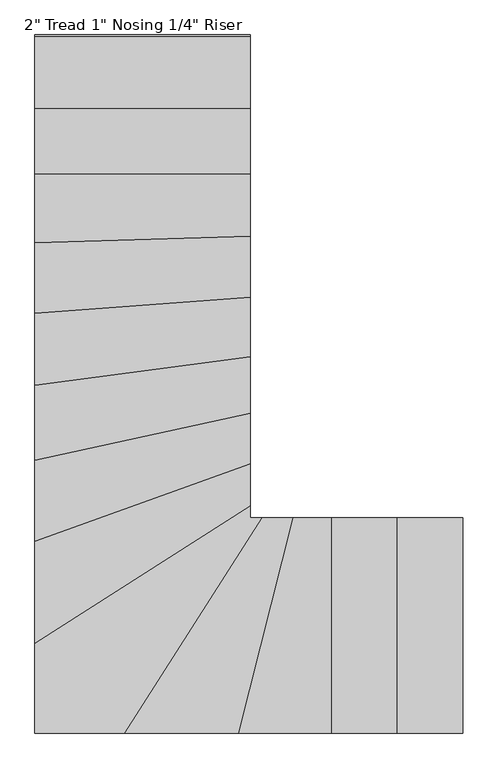
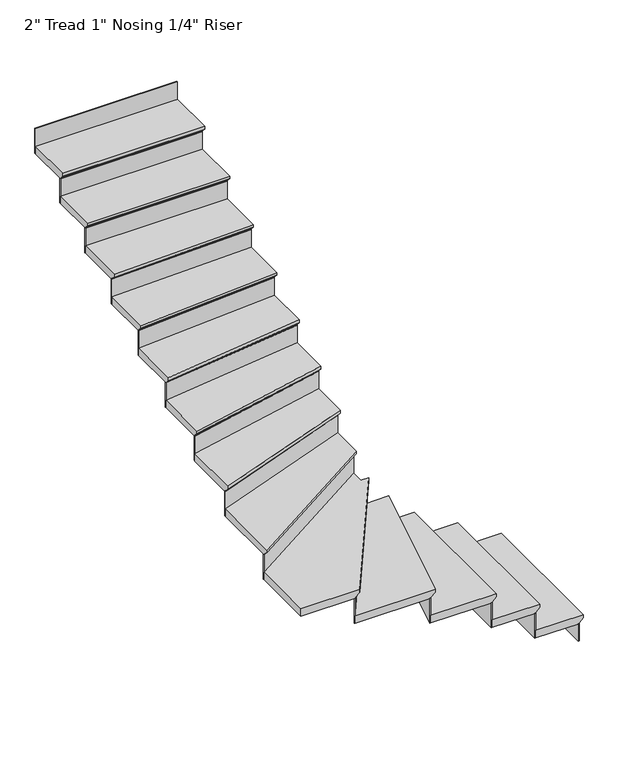
"""IFC4 building model written with IfcOpenShell, lengths in millimetres: stair flight geometry."""

from ifc_helpers import new_model, si_unit, origin, place, context, project, spatial, faceted_brep, source, transform, mapped, element, save


def stair_flight_c47d8ec9(model_context):
    return source(origin(), model_context, "Body", "Brep", [
        faceted_brep([(-4378.4230036, -1246.1564015, 827.6166667), (-4378.4230036, -1246.1564015, 846.6666667), (-4378.4230036, -2160.5564015, 846.6666667), (-4378.4230036, -2160.5564015, 827.6166667), (-4403.8230036, -1246.1564015, 802.2166667), (-4403.8230036, -2160.5564015, 802.2166667), (-4683.2230036, -1246.1564015, 846.6666667), (-4683.2230036, -2160.5564015, 846.6666667), (-4403.8230036, -2160.5564015, 795.8666667), (-4683.2230036, -2160.5564015, 795.8666667), (-4683.2230036, -1246.1564015, 795.8666667), (-4403.8230036, -1246.1564015, 795.8666667)], [[[0, 1, 2, 3]], [[4, 0, 3, 5]], [[2, 1, 6, 7]], [[8, 9, 10, 11]], [[2, 7, 9, 8, 5, 3]], [[8, 11, 4, 5]], [[6, 1, 0, 4, 11, 10]], [[7, 6, 10, 9]]]),
        faceted_brep([(-4403.8230036, -1246.1564015, 795.8666667), (-4403.8230036, -1246.1564015, 677.3333333), (-4410.1730036, -1246.1564015, 677.3333333), (-4410.1730036, -1246.1564015, 795.8666667), (-4403.8230036, -2160.5564015, 795.8666667), (-4410.1730036, -2160.5564015, 795.8666667), (-4410.1730036, -2160.5564015, 677.3333333), (-4403.8230036, -2160.5564015, 677.3333333)], [[[0, 1, 2, 3]], [[4, 5, 6, 7]], [[1, 0, 4, 7]], [[2, 1, 7, 6]], [[3, 2, 6, 5]], [[0, 3, 5, 4]]]),
        faceted_brep([(-4683.2230036, -1246.1564015, 965.2), (-4683.2230036, -1246.1564015, 795.8666667), (-4689.5730036, -1246.1564015, 795.8666667), (-4689.5730036, -1246.1564015, 965.2), (-4683.2230036, -2160.5564015, 965.2), (-4689.5730036, -2160.5564015, 965.2), (-4689.5730036, -2160.5564015, 795.8666667), (-4683.2230036, -2160.5564015, 795.8666667)], [[[0, 1, 2, 3]], [[4, 5, 6, 7]], [[1, 0, 4, 7]], [[2, 1, 7, 6]], [[3, 2, 6, 5]], [[0, 3, 5, 4]]]),
        faceted_brep([(-4657.8230036, -2160.5564015, 1016.0), (-4657.8230036, -1246.1564015, 1016.0), (-4962.6230036, -1246.1564015, 1016.0), (-4962.6230036, -2160.5564015, 1016.0), (-4683.2230036, -2160.5564015, 965.2), (-4962.6230036, -2160.5564015, 965.2), (-4962.6230036, -1246.1564015, 965.2), (-4683.2230036, -1246.1564015, 965.2), (-4683.2230036, -2160.5564015, 971.55), (-4657.8230036, -2160.5564015, 996.95), (-4683.2230036, -1246.1564015, 971.55), (-4657.8230036, -1246.1564015, 996.95)], [[[0, 1, 2, 3]], [[4, 5, 6, 7]], [[0, 3, 5, 4, 8, 9]], [[4, 7, 10, 8]], [[2, 1, 11, 10, 7, 6]], [[3, 2, 6, 5]], [[11, 1, 0, 9]], [[10, 11, 9, 8]]]),
        faceted_brep([(-4962.6230036, -1246.1564015, 1134.5333333), (-4962.6230036, -1246.1564015, 965.2), (-4968.9730036, -1246.1564015, 965.2), (-4968.9730036, -1246.1564015, 1134.5333333), (-4962.6230036, -2160.5564015, 1134.5333333), (-4968.9730036, -2160.5564015, 1134.5333333), (-4968.9730036, -2160.5564015, 965.2), (-4962.6230036, -2160.5564015, 965.2)], [[[0, 1, 2, 3]], [[4, 5, 6, 7]], [[1, 0, 4, 7]], [[2, 1, 7, 6]], [[3, 2, 6, 5]], [[0, 3, 5, 4]]]),
        faceted_brep([(-4937.2230036, -2160.5564015, 1185.3333333), (-4937.2230036, -1246.1564015, 1185.3333333), (-5127.3280374, -1246.1564015, 1185.3333333), (-5358.313714, -2160.5564015, 1185.3333333), (-4962.6230036, -2160.5564015, 1134.5333333), (-5358.313714, -2160.5564015, 1134.5333333), (-5127.3280374, -1246.1564015, 1134.5333333), (-4962.6230036, -1246.1564015, 1134.5333333), (-4962.6230036, -2160.5564015, 1140.8833333), (-4937.2230036, -2160.5564015, 1166.2833333), (-4962.6230036, -1246.1564015, 1140.8833333), (-4937.2230036, -1246.1564015, 1166.2833333)], [[[0, 1, 2, 3]], [[4, 5, 6, 7]], [[0, 3, 5, 4, 8, 9]], [[4, 7, 10, 8]], [[2, 1, 11, 10, 7, 6]], [[3, 2, 6, 5]], [[11, 1, 0, 9]], [[10, 11, 9, 8]]]),
        faceted_brep([(-5127.3280374, -1246.1564015, 1303.8666667), (-5127.3280374, -1246.1564015, 1134.5333333), (-5133.8775055, -1246.1564015, 1134.5333333), (-5133.8775055, -1246.1564015, 1303.8666667), (-5358.313714, -2160.5564015, 1303.8666667), (-5364.8631821, -2160.5564015, 1303.8666667), (-5364.8631821, -2160.5564015, 1134.5333333), (-5358.313714, -2160.5564015, 1134.5333333)], [[[0, 1, 2, 3]], [[4, 5, 6, 7]], [[1, 0, 4, 7]], [[2, 1, 7, 6]], [[3, 2, 6, 5]], [[0, 3, 5, 4]]]),
        faceted_brep([(-5332.1158419, -2160.5564015, 1354.6666667), (-5101.1301653, -1246.1564015, 1354.6666667), (-5261.5956265, -1246.1564015, 1354.6666667), (-5846.1950619, -2160.5564015, 1354.6666667), (-5358.313714, -2160.5564015, 1303.8666667), (-5846.1950619, -2160.5564015, 1303.8666667), (-5261.5956265, -1246.1564015, 1303.8666667), (-5127.3280374, -1246.1564015, 1303.8666667), (-5358.313714, -2160.5564015, 1310.2166667), (-5332.1158419, -2160.5564015, 1335.6166667), (-5127.3280374, -1246.1564015, 1310.2166667), (-5101.1301653, -1246.1564015, 1335.6166667)], [[[0, 1, 2, 3]], [[4, 5, 6, 7]], [[0, 3, 5, 4, 8, 9]], [[4, 7, 10, 8]], [[2, 1, 11, 10, 7, 6]], [[3, 2, 6, 5]], [[11, 1, 0, 9]], [[10, 11, 9, 8]]]),
        faceted_brep([(-5261.5956265, -1246.1564015, 1473.2), (-5261.5956265, -1246.1564015, 1303.8666667), (-5269.1324569, -1246.1564015, 1303.8666667), (-5269.1324569, -1246.1564015, 1473.2), (-5846.1950619, -2160.5564015, 1473.2), (-5853.7318923, -2160.5564015, 1473.2), (-5853.7318923, -2160.5564015, 1303.8666667), (-5846.1950619, -2160.5564015, 1303.8666667)], [[[0, 1, 2, 3]], [[4, 5, 6, 7]], [[1, 0, 4, 7]], [[2, 1, 7, 6]], [[3, 2, 6, 5]], [[0, 3, 5, 4]]]),
        faceted_brep([(-6196.7599931, -1749.696827, 1524.0), (-6196.7599931, -2160.5564015, 1524.0), (-5816.0477402, -2160.5564015, 1524.0), (-5231.4483048, -1246.1564015, 1524.0), (-5282.3599931, -1246.1564015, 1524.0), (-5282.3599931, -1165.0973916, 1524.0), (-6196.7599931, -2160.5564015, 1473.2), (-6196.7599931, -1749.696827, 1473.2), (-5282.3599931, -1165.0973916, 1473.2), (-5282.3599931, -1246.1564015, 1473.2), (-5261.5956265, -1246.1564015, 1473.2), (-5846.1950619, -2160.5564015, 1473.2), (-5261.5956265, -1246.1564015, 1479.55), (-5846.1950619, -2160.5564015, 1479.55), (-5231.4483048, -1246.1564015, 1504.95), (-5816.0477402, -2160.5564015, 1504.95)], [[[0, 1, 2, 3, 4, 5]], [[6, 7, 8, 9, 10, 11]], [[1, 0, 7, 6]], [[11, 10, 12, 13]], [[4, 3, 14, 12, 10, 9]], [[0, 5, 8, 7]], [[14, 3, 2, 15]], [[12, 14, 15, 13]], [[2, 1, 6, 11, 13, 15]], [[5, 4, 9, 8]]]),
        faceted_brep([(-5282.3599931, -1165.0973916, 1642.5333333), (-5282.3599931, -1165.0973916, 1473.2), (-5282.3599931, -1157.5605612, 1473.2), (-5282.3599931, -1157.5605612, 1642.5333333), (-6196.7599931, -1749.696827, 1642.5333333), (-6196.7599931, -1742.1599966, 1642.5333333), (-6196.7599931, -1742.1599966, 1473.2), (-6196.7599931, -1749.696827, 1473.2)], [[[0, 1, 2, 3]], [[4, 5, 6, 7]], [[1, 0, 4, 7]], [[2, 1, 7, 6]], [[3, 2, 6, 5]], [[0, 3, 5, 4]]]),
        faceted_brep([(-6196.7599931, -1779.8441487, 1693.3333333), (-5282.3599931, -1195.2447133, 1693.3333333), (-5282.3599931, -989.1410797, 1693.3333333), (-6196.7599931, -1317.7175845, 1693.3333333), (-6196.7599931, -1749.696827, 1642.5333333), (-6196.7599931, -1317.7175845, 1642.5333333), (-5282.3599931, -989.1410797, 1642.5333333), (-5282.3599931, -1165.0973916, 1642.5333333), (-6196.7599931, -1749.696827, 1648.8833333), (-6196.7599931, -1779.8441487, 1674.2833333), (-5282.3599931, -1165.0973916, 1648.8833333), (-5282.3599931, -1195.2447133, 1674.2833333)], [[[0, 1, 2, 3]], [[4, 5, 6, 7]], [[0, 3, 5, 4, 8, 9]], [[4, 7, 10, 8]], [[2, 1, 11, 10, 7, 6]], [[3, 2, 6, 5]], [[11, 1, 0, 9]], [[10, 11, 9, 8]]]),
        faceted_brep([(-5282.3599931, -989.1410797, 1811.8666667), (-5282.3599931, -989.1410797, 1642.5333333), (-5282.3599931, -982.3935597, 1642.5333333), (-5282.3599931, -982.3935597, 1811.8666667), (-6196.7599931, -1317.7175845, 1811.8666667), (-6196.7599931, -1310.9700645, 1811.8666667), (-6196.7599931, -1310.9700645, 1642.5333333), (-6196.7599931, -1317.7175845, 1642.5333333)], [[[0, 1, 2, 3]], [[4, 5, 6, 7]], [[1, 0, 4, 7]], [[2, 1, 7, 6]], [[3, 2, 6, 5]], [[0, 3, 5, 4]]]),
        faceted_brep([(-6196.7599931, -1344.7076644, 1862.6666667), (-5282.3599931, -1016.1311596, 1862.6666667), (-5282.3599931, -775.0246806, 1862.6666667), (-6196.7599931, -975.0133472, 1862.6666667), (-6196.7599931, -1317.7175845, 1811.8666667), (-6196.7599931, -975.0133472, 1811.8666667), (-5282.3599931, -775.0246806, 1811.8666667), (-5282.3599931, -989.1410797, 1811.8666667), (-6196.7599931, -1317.7175845, 1818.2166667), (-6196.7599931, -1344.7076644, 1843.6166667), (-5282.3599931, -989.1410797, 1818.2166667), (-5282.3599931, -1016.1311596, 1843.6166667)], [[[0, 1, 2, 3]], [[4, 5, 6, 7]], [[0, 3, 5, 4, 8, 9]], [[4, 7, 10, 8]], [[2, 1, 11, 10, 7, 6]], [[3, 2, 6, 5]], [[11, 1, 0, 9]], [[10, 11, 9, 8]]]),
        faceted_brep([(-5282.3599931, -775.0246806, 1981.2), (-5282.3599931, -775.0246806, 1811.8666667), (-5282.3599931, -768.5245811, 1811.8666667), (-5282.3599931, -768.5245811, 1981.2), (-6196.7599931, -975.0133472, 1981.2), (-6196.7599931, -968.5132477, 1981.2), (-6196.7599931, -968.5132477, 1811.8666667), (-6196.7599931, -975.0133472, 1811.8666667)], [[[0, 1, 2, 3]], [[4, 5, 6, 7]], [[1, 0, 4, 7]], [[2, 1, 7, 6]], [[3, 2, 6, 5]], [[0, 3, 5, 4]]]),
        faceted_brep([(-6196.7599931, -1001.0137453, 2032.0), (-5282.3599931, -801.0250787, 2032.0), (-5282.3599931, -535.4776405, 2032.0), (-6196.7599931, -656.5180526, 2032.0), (-6196.7599931, -975.0133472, 1981.2), (-6196.7599931, -656.5180526, 1981.2), (-5282.3599931, -535.4776405, 1981.2), (-5282.3599931, -775.0246806, 1981.2), (-6196.7599931, -975.0133472, 1987.55), (-6196.7599931, -1001.0137453, 2012.95), (-5282.3599931, -775.0246806, 1987.55), (-5282.3599931, -801.0250787, 2012.95)], [[[0, 1, 2, 3]], [[4, 5, 6, 7]], [[0, 3, 5, 4, 8, 9]], [[4, 7, 10, 8]], [[2, 1, 11, 10, 7, 6]], [[3, 2, 6, 5]], [[11, 1, 0, 9]], [[10, 11, 9, 8]]]),
        faceted_brep([(-5282.3599931, -535.4776405, 2150.5333333), (-5282.3599931, -535.4776405, 1981.2), (-5282.3599931, -529.0722492, 1981.2), (-5282.3599931, -529.0722492, 2150.5333333), (-6196.7599931, -656.5180526, 2150.5333333), (-6196.7599931, -650.1126613, 2150.5333333), (-6196.7599931, -650.1126613, 1981.2), (-6196.7599931, -656.5180526, 1981.2)], [[[0, 1, 2, 3]], [[4, 5, 6, 7]], [[1, 0, 4, 7]], [[2, 1, 7, 6]], [[3, 2, 6, 5]], [[0, 3, 5, 4]]]),
        faceted_brep([(-6196.7599931, -682.139618, 2201.3333333), (-5282.3599931, -561.099206, 2201.3333333), (-5282.3599931, -282.9309158, 2201.3333333), (-6196.7599931, -350.56912, 2201.3333333), (-6196.7599931, -656.5180526, 2150.5333333), (-6196.7599931, -350.56912, 2150.5333333), (-5282.3599931, -282.9309158, 2150.5333333), (-5282.3599931, -535.4776405, 2150.5333333), (-6196.7599931, -656.5180526, 2156.8833333), (-6196.7599931, -682.139618, 2182.2833333), (-5282.3599931, -535.4776405, 2156.8833333), (-5282.3599931, -561.099206, 2182.2833333)], [[[0, 1, 2, 3]], [[4, 5, 6, 7]], [[0, 3, 5, 4, 8, 9]], [[4, 7, 10, 8]], [[2, 1, 11, 10, 7, 6]], [[3, 2, 6, 5]], [[11, 1, 0, 9]], [[10, 11, 9, 8]]]),
        faceted_brep([(-5282.3599931, -282.9309158, 2319.8666667), (-5282.3599931, -282.9309158, 2150.5333333), (-5282.3599931, -276.5635673, 2150.5333333), (-5282.3599931, -276.5635673, 2319.8666667), (-6196.7599931, -350.56912, 2319.8666667), (-6196.7599931, -344.2017715, 2319.8666667), (-6196.7599931, -344.2017715, 2150.5333333), (-6196.7599931, -350.56912, 2150.5333333)], [[[0, 1, 2, 3]], [[4, 5, 6, 7]], [[1, 0, 4, 7]], [[2, 1, 7, 6]], [[3, 2, 6, 5]], [[0, 3, 5, 4]]]),
        faceted_brep([(-6196.7599931, -376.0385141, 2370.6666667), (-5282.3599931, -308.4003099, 2370.6666667), (-5282.3599931, -22.8518026, 2370.6666667), (-6196.7599931, -51.9612867, 2370.6666667), (-6196.7599931, -350.56912, 2319.8666667), (-6196.7599931, -51.9612867, 2319.8666667), (-5282.3599931, -22.8518026, 2319.8666667), (-5282.3599931, -282.9309158, 2319.8666667), (-6196.7599931, -350.56912, 2326.2166667), (-6196.7599931, -376.0385141, 2351.6166667), (-5282.3599931, -282.9309158, 2326.2166667), (-5282.3599931, -308.4003099, 2351.6166667)], [[[0, 1, 2, 3]], [[4, 5, 6, 7]], [[0, 3, 5, 4, 8, 9]], [[4, 7, 10, 8]], [[2, 1, 11, 10, 7, 6]], [[3, 2, 6, 5]], [[11, 1, 0, 9]], [[10, 11, 9, 8]]]),
        faceted_brep([(-5282.3599931, -22.8518026, 2489.2), (-5282.3599931, -22.8518026, 2319.8666667), (-5282.3599931, -16.4985857, 2319.8666667), (-5282.3599931, -16.4985857, 2489.2), (-6196.7599931, -51.9612867, 2489.2), (-6196.7599931, -45.6080698, 2489.2), (-6196.7599931, -45.6080698, 2319.8666667), (-6196.7599931, -51.9612867, 2319.8666667)], [[[0, 1, 2, 3]], [[4, 5, 6, 7]], [[1, 0, 4, 7]], [[2, 1, 7, 6]], [[3, 2, 6, 5]], [[0, 3, 5, 4]]]),
        faceted_brep([(-6196.7599931, -77.3741541, 2540.0), (-5282.3599931, -48.26467, 2540.0), (-5282.3599931, 241.980588, 2540.0), (-6196.7599931, 241.980588, 2540.0), (-6196.7599931, -51.9612867, 2489.2), (-6196.7599931, 241.980588, 2489.2), (-5282.3599931, 241.980588, 2489.2), (-5282.3599931, -22.8518026, 2489.2), (-6196.7599931, -51.9612867, 2495.55), (-6196.7599931, -77.3741541, 2520.95), (-5282.3599931, -22.8518026, 2495.55), (-5282.3599931, -48.26467, 2520.95)], [[[0, 1, 2, 3]], [[4, 5, 6, 7]], [[0, 3, 5, 4, 8, 9]], [[4, 7, 10, 8]], [[2, 1, 11, 10, 7, 6]], [[3, 2, 6, 5]], [[11, 1, 0, 9]], [[10, 11, 9, 8]]]),
        faceted_brep([(-5282.3599931, 241.980588, 2658.5333333), (-5282.3599931, 241.980588, 2489.2), (-5282.3599931, 248.330588, 2489.2), (-5282.3599931, 248.330588, 2658.5333333), (-6196.7599931, 241.980588, 2658.5333333), (-6196.7599931, 248.330588, 2658.5333333), (-6196.7599931, 248.330588, 2489.2), (-6196.7599931, 241.980588, 2489.2)], [[[0, 1, 2, 3]], [[4, 5, 6, 7]], [[1, 0, 4, 7]], [[2, 1, 7, 6]], [[3, 2, 6, 5]], [[0, 3, 5, 4]]]),
        faceted_brep([(-6196.7599931, 216.580588, 2709.3333333), (-5282.3599931, 216.580588, 2709.3333333), (-5282.3599931, 521.380588, 2709.3333333), (-6196.7599931, 521.380588, 2709.3333333), (-6196.7599931, 241.980588, 2658.5333333), (-6196.7599931, 521.380588, 2658.5333333), (-5282.3599931, 521.380588, 2658.5333333), (-5282.3599931, 241.980588, 2658.5333333), (-6196.7599931, 241.980588, 2664.8833333), (-6196.7599931, 216.580588, 2690.2833333), (-5282.3599931, 241.980588, 2664.8833333), (-5282.3599931, 216.580588, 2690.2833333)], [[[0, 1, 2, 3]], [[4, 5, 6, 7]], [[0, 3, 5, 4, 8, 9]], [[4, 7, 10, 8]], [[2, 1, 11, 10, 7, 6]], [[3, 2, 6, 5]], [[11, 1, 0, 9]], [[10, 11, 9, 8]]]),
        faceted_brep([(-5282.3599931, 521.380588, 2827.8666667), (-5282.3599931, 521.380588, 2658.5333333), (-5282.3599931, 527.730588, 2658.5333333), (-5282.3599931, 527.730588, 2827.8666667), (-6196.7599931, 521.380588, 2827.8666667), (-6196.7599931, 527.730588, 2827.8666667), (-6196.7599931, 527.730588, 2658.5333333), (-6196.7599931, 521.380588, 2658.5333333)], [[[0, 1, 2, 3]], [[4, 5, 6, 7]], [[1, 0, 4, 7]], [[2, 1, 7, 6]], [[3, 2, 6, 5]], [[0, 3, 5, 4]]]),
        faceted_brep([(-5282.3599931, 800.780588, 2997.2), (-5282.3599931, 800.780588, 2827.8666667), (-5282.3599931, 807.130588, 2827.8666667), (-5282.3599931, 807.130588, 2997.2), (-6196.7599931, 800.780588, 2997.2), (-6196.7599931, 807.130588, 2997.2), (-6196.7599931, 807.130588, 2827.8666667), (-6196.7599931, 800.780588, 2827.8666667)], [[[0, 1, 2, 3]], [[4, 5, 6, 7]], [[1, 0, 4, 7]], [[2, 1, 7, 6]], [[3, 2, 6, 5]], [[0, 3, 5, 4]]]),
        faceted_brep([(-6196.7599931, 495.980588, 2878.6666667), (-5282.3599931, 495.980588, 2878.6666667), (-5282.3599931, 800.780588, 2878.6666667), (-6196.7599931, 800.780588, 2878.6666667), (-6196.7599931, 521.380588, 2827.8666667), (-6196.7599931, 800.780588, 2827.8666667), (-5282.3599931, 800.780588, 2827.8666667), (-5282.3599931, 521.380588, 2827.8666667), (-6196.7599931, 521.380588, 2834.2166667), (-6196.7599931, 495.980588, 2859.6166667), (-5282.3599931, 521.380588, 2834.2166667), (-5282.3599931, 495.980588, 2859.6166667)], [[[0, 1, 2, 3]], [[4, 5, 6, 7]], [[0, 3, 5, 4, 8, 9]], [[4, 7, 10, 8]], [[2, 1, 11, 10, 7, 6]], [[3, 2, 6, 5]], [[11, 1, 0, 9]], [[10, 11, 9, 8]]]),
    ])


if __name__ == "__main__":
    model = new_model("IFC4")
    model_context = context("Model", 3, world=origin())
    ifc_project = project(units=[si_unit("LENGTHUNIT", "METRE", prefix="MILLI")], contexts=[model_context])
    site = spatial("IfcSite", under=ifc_project)
    building = spatial("IfcBuilding", under=site)
    placement = place(None, origin())
    stair_flight_shape = stair_flight_c47d8ec9(model_context)
    element("IfcStairFlight", 1, ObjectType="2\" Tread 1\" Nosing 1/4\" Riser", at=placement, inside=building, context=model_context, shape_type="MappedRepresentation", body=[
        mapped(stair_flight_shape, transform((0.0, 0.0, 0.0), x_axis=(1.0, 0.0, 0.0), y_axis=(0.0, 1.0, 0.0), z_axis=(0.0, 0.0, 1.0))),
    ])
    save(model, "model.ifc")
